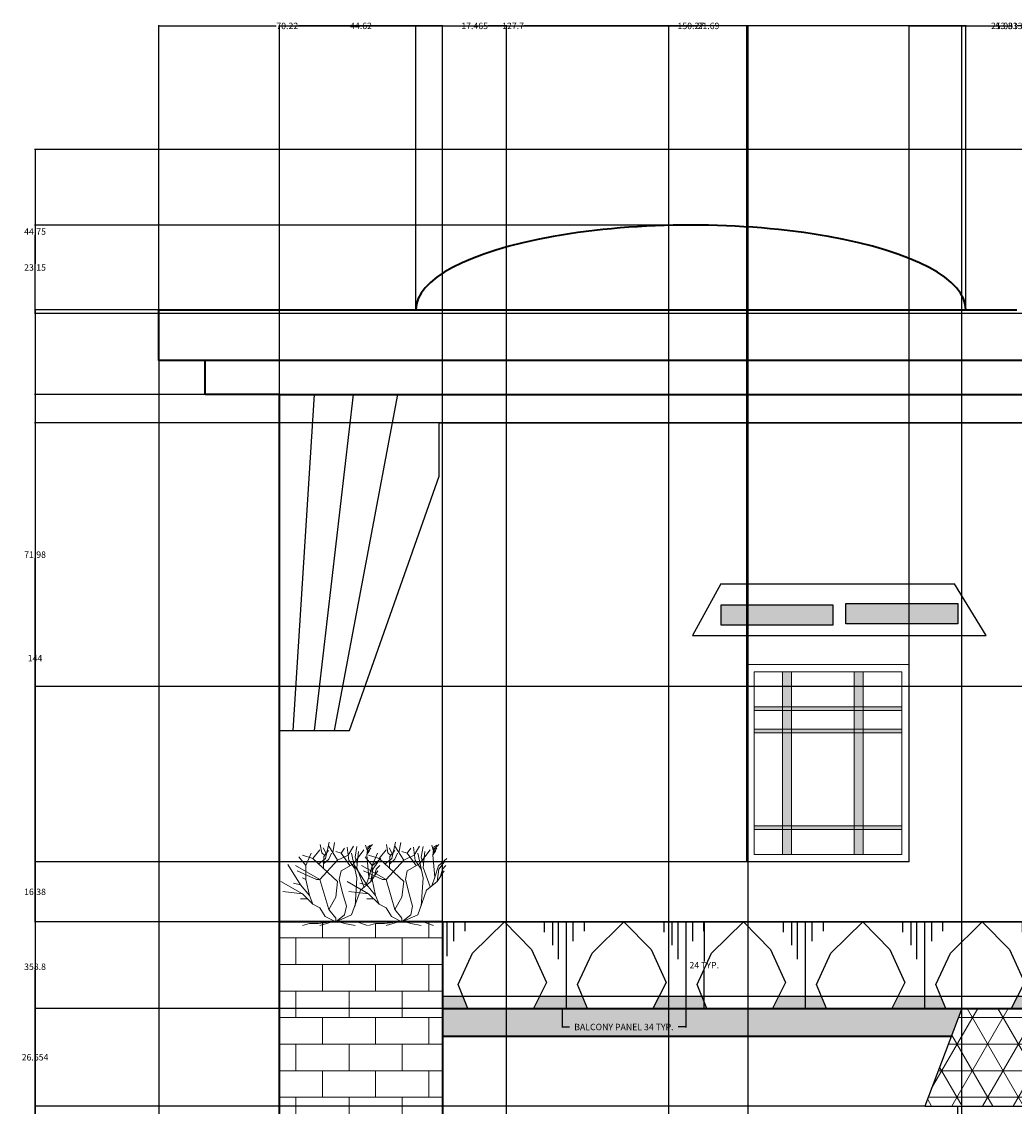
# Model space of a CAD drawing. Units: inches. Extents: x -17 to 741, y 7 to 490.
# Tile 2 of 8: x -17 to 254, y 193 to 490. Entities that reach past the tile are written whole.
import ezdxf

# ---------------------------------------------------------------- set-up
doc = ezdxf.new("R2010")
doc.units = ezdxf.units.IN
doc.header["$MEASUREMENT"] = 0
for name, color, linetype, lineweight in [('A-ANNO-DIMS', 2, 'Continuous', 18), ('A-ELEV-PATT', 252, 'Continuous', 13), ('A-FLOR-RAIL', 7, 'Continuous', 25), ('A-GLAZ', 4, 'Continuous', 18), ('A-ROOF', 7, 'Continuous', 35), ('A-ROOF-CNPE', 7, 'Continuous', 25), ('A-ROOF-PATT', 8, 'Continuous', 13), ('A-WALL', 7, 'Continuous', 35), ('A-WALL-PATT', 8, 'Continuous', 13), ('A-WALL-TRIM', 7, 'Continuous', 25), ('L-PLNT', 3, 'Continuous', 18)]:
    doc.layers.add(name, color=color, linetype=linetype, lineweight=lineweight)
doc.styles.get("Standard").update_dxf_attribs({"font": 'arial.ttf'})
doc.dimstyles.get("Standard").update_dxf_attribs({"dimtxt": 1.75, "dimasz": 0.18, "dimexe": 0.18, "dimexo": 0.0625, "dimgap": 0.09, "dimtad": 0, "dimtih": 1, "dimtoh": 1, "dimdec": 4, "dimzin": 0, "dimdsep": 46, "dimlunit": 4, "dimtxsty": 'Standard', "dimcen": 0.09, "dimadec": 0, "dimazin": 0, "dimtfac": 1, "dimtdec": 4, "dimtofl": 0, "dimtmove": 0, "dimatfit": 3, "dimfxl": 1, "dimtolj": 1, "dimtzin": 0, "dimarcsym": 0})

# ---------------------------------------------------------------- blocks, each defined once
blk = doc.blocks.new('Shrub - elevation')
for p, q in [((-12.471, 19.775), (-12.898, 22.044)), ((-11.28, 19.619), (-12.104, 21.184)), ((-11.433, 18.289), (-10.457, 22.749)), ((-8.16, 17.76), (-10.56, 21.6)), ((-9.48, 19.775), (-8.992, 22.592)), ((-7.2, 19.68), (-6.24, 21.12)), ((-5.086, 17.741), (-5.513, 21.34)), ((-5.28, 19.2), (-3.84, 21.6)), ((-3.377, 18.602), (-2.888, 21.575)), ((-0.508, 21.888), (-0.081, 20.558)), ((-0.203, 19.149), (0.102, 21.34)), ((-0.02, 20.01), (0.896, 21.105)), ((0.041, 20.714), (1.384, 22.044)), ((0.102, 21.34), (0.835, 21.888)), ((-16.8, 16.32), (-18.72, 18.72)), ((-14.88, 18.24), (-17.76, 19.2)), ((-16.8, 16.32), (-15.36, 19.68)), ((-14.88, 18.24), (-12.96, 20.64)), ((-8.16, 12), (-14.88, 18.24)), ((-13.325, 16.724), (-11.433, 18.289)), ((-11.677, 19.071), (-12.471, 19.775)), ((-12.043, 15.628), (-11.921, 18.836)), ((-11.982, 16.802), (-10.579, 18.054)), ((-11.921, 18.836), (-10.64, 20.401)), ((-10.579, 18.054), (-9.846, 19.697)), ((-7.2, 19.68), (-8.64, 20.16)), ((-8.16, 17.76), (-5.28, 19.2)), ((-4.8, 16.32), (-7.2, 19.68)), ((-3.377, 15.315), (-5.086, 17.819)), ((-2.88, 12.96), (-4.32, 19.68)), ((-3.84, 16.8), (-0.96, 20.64)), ((-2.766, 16.802), (-3.377, 18.602)), ((-2.88, 15.84), (-2.4, 20.16)), ((0.346, 13.203), (-0.203, 19.149)), ((-0.142, 19.384), (0.59, 20.401)), ((1.323, 16.254), (3.642, 18.289)), ((-18.24, 11.04), (-21.755, 16.655)), ((-12.96, 12.48), (-19.68, 16.32)), ((-13.92, 12.48), (-19.2, 14.88)), ((-16.8, 12.48), (-16.8, 16.32)), ((-12.96, 12.48), (-8.16, 17.76)), ((-7.68, 12.48), (-7.2, 14.88)), ((-7.2, 14.88), (-3.84, 16.8)), ((-0.96, 10.56), (-2.88, 15.84)), ((0.346, 13.203), (1.323, 16.254)), ((0.96, 12), (1.44, 15.36)), ((0.96, 12), (2.88, 14.88)), ((1.44, 15.36), (2.88, 17.28)), ((1.92, 13.44), (2.4, 15.36)), ((2.4, 15.36), (3.36, 16.32)), ((-17.76, 8.64), (-23.663, 11.961)), ((-16.8, 12.48), (-17.76, 12.96)), ((-15.84, 8.16), (-16.8, 12.48)), ((-12.96, 12.48), (-13.92, 12.48)), ((-10.56, 4.32), (-12.96, 12.48)), ((-8.64, 7.68), (-8.16, 12)), ((-6.72, 8.64), (-7.68, 12.48)), ((-3.36, 5.28), (-2.88, 12.96)), ((-1.92, 9.6), (0.96, 12)), ((-0.48, 10.8), (0.346, 13.203)), ((-17.76, 8.64), (-23.128, 9.222)), ((-18.24, 11.04), (-20.16, 11.52)), ((-15.84, 8.16), (-18.24, 11.04)), ((-4.32, 2.88), (-1.92, 9.6)), ((-16.32, 7.2), (-18.24, 7.2)), ((-14.88, 5.76), (-17.76, 8.64)), ((-14.88, 5.76), (-15.84, 8.16)), ((-10.56, 4.32), (-8.64, 7.68)), ((-5.76, 5.28), (-6.72, 8.64)), ((-12.96, 4.8), (-14.88, 5.76)), ((-11.52, 2.4), (-12.96, 4.8)), ((-8.64, 1.92), (-10.56, 4.32)), ((-6.24, 2.88), (-5.76, 5.28)), ((-15.84, 0.48), (-17.76, 0)), ((-13.44, 0.48), (-15.84, 0.48)), ((-9.6, 0.96), (-13.44, 0.48)), ((-9.6, 0.96), (-12.96, 0)), ((-8.64, 0.96), (-11.52, 2.4)), ((-9.6, 0.96), (-7.68, 0.96)), ((-8.64, 0.96), (-4.32, 2.88)), ((-8.64, 0.96), (-6.24, 2.88)), ((-8.64, 0.96), (-8.64, 1.92)), ((-8.64, 0.96), (-2.88, 0.96)), ((-7.68, 0.96), (-6.24, 0.48)), ((-6.24, 0.48), (-3.36, 0)), ((-2.88, 0.96), (0, 0))]:
    blk.add_line(p, q)
blk = doc.blocks.new('BALCONY-POINTED-PANEL')
for p, q in [((0, 23.66), (33.75, 23.66)), ((1.12, 23.66), (1.12, 14.33)), ((2.97, 23.66), (2.97, 18.36)), ((6.01, 23.66), (6.01, 21.09)), ((27.76, 23.66), (27.76, 20.83)), ((29.99, 23.66), (29.99, 17.32)), ((31.57, 23.66), (31.57, 13.51)), ((33.75, 23.66), (33.75, 0))]:
    blk.add_line(p, q)
blk.add_lwpolyline([(6.92, 0), (4.23, 6.57), (8.17, 15.14), (16.88, 23.66), (24.3, 16.07), (28.38, 7.1), (24.8, 0)])
blk = doc.blocks.new('WIN-ELEV-DIVIDED')
for p, q in [((9.78, 51.92), (9.78, 2)), ((12.23, 51.92), (12.23, 2)), ((29.29, 51.92), (29.29, 2)), ((31.75, 51.92), (31.75, 2)), ((2, 42.35), (42.31, 42.35)), ((2, 41.35), (42.31, 41.35)), ((2, 36.22), (42.31, 36.22)), ((2, 35.22), (42.31, 35.22)), ((2, 9.85), (42.31, 9.85)), ((2, 8.85), (42.31, 8.85))]:
    blk.add_line(p, q)
for points in [[(0, 0), (44.31, 0), (44.31, 53.92), (0, 53.92)], [(2, 2), (42.31, 2), (42.31, 51.92), (2, 51.92)]]:
    blk.add_lwpolyline(points, close=True)
blk = doc.blocks.new('*D15')
at = {"layer": 'A-ANNO-DIMS', "color": 0, "lineweight": -2, "transparency": 16777216}
for p, q in [((130.71, 219.95), (130.71, 214.77)), ((164.46, 219.95), (164.46, 214.77)), ((130.89, 214.95), (132.74, 214.95)), ((164.28, 214.95), (162.42, 214.95))]:
    blk.add_line(p, q, dxfattribs=at)
at = {"layer": 'A-ANNO-DIMS', "color": 0, "transparency": 16777216}
for points in [[(130.89, 214.98), (130.89, 214.92), (130.71, 214.95)], [(164.28, 214.98), (164.28, 214.92), (164.46, 214.95)]]:
    blk.add_solid(points, dxfattribs=at)
at = {"layer": 'Defpoints', "color": 0, "transparency": 16777216}
for p in [(130.71, 220.01), (164.46, 220.01), (164.46, 214.95)]:
    blk.add_point(p, dxfattribs=at)
at = {"layer": 'A-ANNO-DIMS', "color": 0, "transparency": 16777216, "insert": (147.58, 214.95), "char_height": 1.75, "attachment_point": 5}
blk.add_mtext('\\A1;BALCONY PANEL 34 TYP.', dxfattribs=at)
blk = doc.blocks.new('*D16')
at = {"layer": 'A-ANNO-DIMS', "color": 0, "lineweight": -2, "transparency": 16777216}
for p, q in [((164.52, 243.67), (169.7, 243.67)), ((169.52, 243.49), (169.52, 232.81)), ((169.52, 220.19), (169.52, 230.87)), ((164.52, 220.01), (169.7, 220.01))]:
    blk.add_line(p, q, dxfattribs=at)
at = {"layer": 'A-ANNO-DIMS', "color": 0, "transparency": 16777216}
for points in [[(169.49, 243.49), (169.55, 243.49), (169.52, 243.67)], [(169.49, 220.19), (169.55, 220.19), (169.52, 220.01)]]:
    blk.add_solid(points, dxfattribs=at)
at = {"layer": 'Defpoints', "color": 0, "transparency": 16777216}
for p in [(164.46, 243.67), (169.52, 243.67), (164.46, 220.01)]:
    blk.add_point(p, dxfattribs=at)
at = {"layer": 'A-ANNO-DIMS', "color": 0, "transparency": 16777216, "insert": (169.52, 231.84), "char_height": 1.75, "attachment_point": 5}
blk.add_mtext('\\A1;24 TYP.', dxfattribs=at)
blk = doc.blocks.new('*D37')
at = {"layer": 'A-ANNO-DIMS', "color": 0, "lineweight": -2, "transparency": 16777216}
for p, q in [((20.52, 396.95), (20.52, 14.58)), ((553.43, 51.95), (553.43, 14.58)), ((20.7, 14.76), (283.93, 14.76)), ((553.25, 14.76), (290.02, 14.76))]:
    blk.add_line(p, q, dxfattribs=at)
at = {"layer": 'A-ANNO-DIMS', "color": 0, "transparency": 16777216}
for points in [[(20.7, 14.79), (20.7, 14.73), (20.52, 14.76)], [(553.25, 14.79), (553.25, 14.73), (553.43, 14.76)]]:
    blk.add_solid(points, dxfattribs=at)
at = {"layer": 'Defpoints', "color": 0, "transparency": 16777216}
for p in [(20.52, 397.01), (553.43, 52.01), (553.43, 14.76)]:
    blk.add_point(p, dxfattribs=at)
at = {"layer": 'A-ANNO-DIMS', "color": 0, "transparency": 16777216, "insert": (286.97, 14.76), "char_height": 1.75, "attachment_point": 5}
blk.add_mtext('\\A1;532.9', dxfattribs=at)
blk = doc.blocks.new('*D39')
at = {"layer": 'A-ANNO-DIMS', "color": 0, "lineweight": -2, "transparency": 16777216}
for p, q in [((20.45, 410.82), (-13.46, 410.82)), ((-13.28, 410.64), (-13.28, 232.4)), ((-13.28, 52.19), (-13.28, 230.43)), ((53.4, 52.01), (-13.46, 52.01))]:
    blk.add_line(p, q, dxfattribs=at)
at = {"layer": 'A-ANNO-DIMS', "color": 0, "transparency": 16777216}
for points in [[(-13.31, 410.64), (-13.25, 410.64), (-13.28, 410.82)], [(-13.31, 52.19), (-13.25, 52.19), (-13.28, 52.01)]]:
    blk.add_solid(points, dxfattribs=at)
at = {"layer": 'Defpoints', "color": 0, "transparency": 16777216}
for p in [(-13.28, 410.82), (20.52, 410.82), (53.46, 52.01)]:
    blk.add_point(p, dxfattribs=at)
at = {"layer": 'A-ANNO-DIMS', "color": 0, "transparency": 16777216, "insert": (-13.28, 231.41), "char_height": 1.75, "attachment_point": 5}
blk.add_mtext('\\A1;358.8', dxfattribs=at)
blk = doc.blocks.new('*D40')
at = {"layer": 'A-ANNO-DIMS', "color": 0, "lineweight": -2, "transparency": 16777216}
for p, q in [((165.8, 433.97), (-13.46, 433.97)), ((-13.28, 433.79), (-13.28, 423.38)), ((-13.28, 411), (-13.28, 421.41)), ((90.67, 410.82), (-13.46, 410.82))]:
    blk.add_line(p, q, dxfattribs=at)
at = {"layer": 'A-ANNO-DIMS', "color": 0, "transparency": 16777216}
for points in [[(-13.31, 433.79), (-13.25, 433.79), (-13.28, 433.97)], [(-13.31, 411), (-13.25, 411), (-13.28, 410.82)]]:
    blk.add_solid(points, dxfattribs=at)
at = {"layer": 'Defpoints', "color": 0, "transparency": 16777216}
for p in [(-13.28, 433.97), (165.87, 433.97), (90.73, 410.82)]:
    blk.add_point(p, dxfattribs=at)
at = {"layer": 'A-ANNO-DIMS', "color": 0, "transparency": 16777216, "insert": (-13.28, 422.39), "char_height": 1.75, "attachment_point": 5}
blk.add_mtext('\\A1;23.15', dxfattribs=at)
blk = doc.blocks.new('*D41')
at = {"layer": 'A-ANNO-DIMS', "color": 0, "lineweight": -2, "transparency": 16777216}
for p, q in [((20.52, 410.88), (20.52, 488.55)), ((20.7, 488.37), (52.6, 488.37)), ((90.55, 488.37), (58.65, 488.37)), ((90.73, 410.88), (90.73, 488.55))]:
    blk.add_line(p, q, dxfattribs=at)
at = {"layer": 'A-ANNO-DIMS', "color": 0, "transparency": 16777216}
for points in [[(20.7, 488.4), (20.7, 488.34), (20.52, 488.37)], [(90.55, 488.4), (90.55, 488.34), (90.73, 488.37)]]:
    blk.add_solid(points, dxfattribs=at)
at = {"layer": 'Defpoints', "color": 0, "transparency": 16777216}
for p in [(90.73, 488.37), (20.52, 410.82), (90.73, 410.82)]:
    blk.add_point(p, dxfattribs=at)
at = {"layer": 'A-ANNO-DIMS', "color": 0, "transparency": 16777216, "insert": (55.62, 488.37), "char_height": 1.75, "attachment_point": 5}
blk.add_mtext('\\A1;70.22', dxfattribs=at)
blk = doc.blocks.new('*D42')
at = {"layer": 'A-ANNO-DIMS', "color": 0, "lineweight": -2, "transparency": 16777216}
for p, q in [((90.73, 410.88), (90.73, 488.55)), ((90.91, 488.37), (162.23, 488.37)), ((240.82, 488.37), (169.51, 488.37)), ((241, 410.88), (241, 488.55))]:
    blk.add_line(p, q, dxfattribs=at)
at = {"layer": 'A-ANNO-DIMS', "color": 0, "transparency": 16777216}
for points in [[(90.91, 488.4), (90.91, 488.34), (90.73, 488.37)], [(240.82, 488.4), (240.82, 488.34), (241, 488.37)]]:
    blk.add_solid(points, dxfattribs=at)
at = {"layer": 'Defpoints', "color": 0, "transparency": 16777216}
for p in [(241, 488.37), (90.73, 410.82), (241, 410.82)]:
    blk.add_point(p, dxfattribs=at)
at = {"layer": 'A-ANNO-DIMS', "color": 0, "transparency": 16777216, "insert": (165.87, 488.37), "char_height": 1.75, "attachment_point": 5}
blk.add_mtext('\\A1;150.27', dxfattribs=at)
blk = doc.blocks.new('*D43')
at = {"layer": 'A-ANNO-DIMS', "color": 0, "lineweight": -2, "transparency": 16777216}
for p, q in [((241, 410.88), (241, 488.55)), ((241.18, 488.37), (247.8, 488.37)), ((261.9, 488.37), (255.28, 488.37)), ((262.08, 409.88), (262.08, 488.55))]:
    blk.add_line(p, q, dxfattribs=at)
at = {"layer": 'A-ANNO-DIMS', "color": 0, "transparency": 16777216}
for points in [[(241.18, 488.4), (241.18, 488.34), (241, 488.37)], [(261.9, 488.4), (261.9, 488.34), (262.08, 488.37)]]:
    blk.add_solid(points, dxfattribs=at)
at = {"layer": 'Defpoints', "color": 0, "transparency": 16777216}
for p in [(262.08, 488.37), (241, 410.82), (262.08, 409.82)]:
    blk.add_point(p, dxfattribs=at)
at = {"layer": 'A-ANNO-DIMS', "color": 0, "transparency": 16777216, "insert": (251.54, 488.37), "char_height": 1.75, "attachment_point": 5}
blk.add_mtext('\\A1;21.083', dxfattribs=at)
blk = doc.blocks.new('*D45')
at = {"layer": 'A-ANNO-DIMS', "color": 0, "lineweight": -2, "transparency": 16777216}
for p, q in [((341.71, 454.57), (-13.46, 454.57)), ((-13.28, 454.39), (-13.28, 433.18)), ((-13.28, 410), (-13.28, 431.22)), ((262.02, 409.82), (-13.46, 409.82))]:
    blk.add_line(p, q, dxfattribs=at)
at = {"layer": 'A-ANNO-DIMS', "color": 0, "transparency": 16777216}
for points in [[(-13.31, 454.39), (-13.25, 454.39), (-13.28, 454.57)], [(-13.31, 410), (-13.25, 410), (-13.28, 409.82)]]:
    blk.add_solid(points, dxfattribs=at)
at = {"layer": 'Defpoints', "color": 0, "transparency": 16777216}
for p in [(-13.28, 454.57), (341.77, 454.57), (262.08, 409.82)]:
    blk.add_point(p, dxfattribs=at)
at = {"layer": 'A-ANNO-DIMS', "color": 0, "transparency": 16777216, "insert": (-13.28, 432.2), "char_height": 1.75, "attachment_point": 5}
blk.add_mtext('\\A1;44.75', dxfattribs=at)
blk = doc.blocks.new('*D47')
at = {"layer": 'A-ANNO-DIMS', "color": 0, "lineweight": -2, "transparency": 16777216}
for p, q in [((493.03, 379.95), (-13.46, 379.95)), ((-13.28, 379.77), (-13.28, 344.94)), ((-13.28, 308.15), (-13.28, 342.97)), ((553.37, 307.97), (-13.46, 307.97))]:
    blk.add_line(p, q, dxfattribs=at)
at = {"layer": 'A-ANNO-DIMS', "color": 0, "transparency": 16777216}
for points in [[(-13.31, 379.77), (-13.25, 379.77), (-13.28, 379.95)], [(-13.31, 308.15), (-13.25, 308.15), (-13.28, 307.97)]]:
    blk.add_solid(points, dxfattribs=at)
at = {"layer": 'Defpoints', "color": 0, "transparency": 16777216}
for p in [(493.1, 379.95), (-13.28, 307.97), (553.43, 307.97)]:
    blk.add_point(p, dxfattribs=at)
at = {"layer": 'A-ANNO-DIMS', "color": 0, "transparency": 16777216, "insert": (-13.28, 343.96), "char_height": 1.75, "attachment_point": 5}
blk.add_mtext('\\A1;71.98', dxfattribs=at)
blk = doc.blocks.new('*D49')
at = {"layer": 'A-ANNO-DIMS', "color": 0, "lineweight": -2, "transparency": 16777216}
for p, q in [((53.4, 243.67), (-13.46, 243.67)), ((-13.28, 243.49), (-13.28, 160.82)), ((-13.28, 76.19), (-13.28, 158.86)), ((53.4, 76.01), (-13.46, 76.01))]:
    blk.add_line(p, q, dxfattribs=at)
at = {"layer": 'A-ANNO-DIMS', "color": 0, "transparency": 16777216}
for points in [[(-13.31, 243.49), (-13.25, 243.49), (-13.28, 243.67)], [(-13.31, 76.19), (-13.25, 76.19), (-13.28, 76.01)]]:
    blk.add_solid(points, dxfattribs=at)
at = {"layer": 'Defpoints', "color": 0, "transparency": 16777216}
for p in [(-13.28, 243.67), (53.46, 243.67), (53.46, 76.01)]:
    blk.add_point(p, dxfattribs=at)
at = {"layer": 'A-ANNO-DIMS', "color": 0, "transparency": 16777216, "insert": (-13.28, 159.84), "char_height": 1.75, "attachment_point": 5}
blk.add_mtext('\\A1;167.66', dxfattribs=at)
blk = doc.blocks.new('*D50')
at = {"layer": 'A-ANNO-DIMS', "color": 0, "lineweight": -2, "transparency": 16777216}
for p, q in [((53.4, 387.67), (-13.46, 387.67)), ((-13.28, 387.49), (-13.28, 316.64)), ((-13.28, 243.85), (-13.28, 314.7)), ((53.4, 243.67), (-13.46, 243.67))]:
    blk.add_line(p, q, dxfattribs=at)
at = {"layer": 'A-ANNO-DIMS', "color": 0, "transparency": 16777216}
for points in [[(-13.31, 387.49), (-13.25, 387.49), (-13.28, 387.67)], [(-13.31, 243.85), (-13.25, 243.85), (-13.28, 243.67)]]:
    blk.add_solid(points, dxfattribs=at)
at = {"layer": 'Defpoints', "color": 0, "transparency": 16777216}
for p in [(-13.28, 387.67), (53.46, 387.67), (53.46, 243.67)]:
    blk.add_point(p, dxfattribs=at)
at = {"layer": 'A-ANNO-DIMS', "color": 0, "transparency": 16777216, "insert": (-13.28, 315.67), "char_height": 1.75, "attachment_point": 5}
blk.add_mtext('\\A1;144', dxfattribs=at)
blk = doc.blocks.new('*D51')
at = {"layer": 'A-ANNO-DIMS', "color": 0, "lineweight": -2, "transparency": 16777216}
for p, q in [((53.46, 52.07), (53.46, 488.55)), ((53.64, 488.37), (72.7, 488.37)), ((97.89, 488.37), (78.84, 488.37)), ((98.07, 52.07), (98.07, 488.55))]:
    blk.add_line(p, q, dxfattribs=at)
at = {"layer": 'A-ANNO-DIMS', "color": 0, "transparency": 16777216}
for points in [[(53.64, 488.4), (53.64, 488.34), (53.46, 488.37)], [(97.89, 488.4), (97.89, 488.34), (98.07, 488.37)]]:
    blk.add_solid(points, dxfattribs=at)
at = {"layer": 'Defpoints', "color": 0, "transparency": 16777216}
for p in [(98.07, 488.37), (53.46, 52.01), (98.07, 52.01)]:
    blk.add_point(p, dxfattribs=at)
at = {"layer": 'A-ANNO-DIMS', "color": 0, "transparency": 16777216, "insert": (75.77, 488.37), "char_height": 1.75, "attachment_point": 5}
blk.add_mtext('\\A1;44.62', dxfattribs=at)
blk = doc.blocks.new('*D52')
at = {"layer": 'A-ANNO-DIMS', "color": 0, "lineweight": -2, "transparency": 16777216}
for p, q in [((239.94, 113.25), (239.94, 488.55)), ((240.12, 488.37), (253.76, 488.37)), ((273.51, 488.37), (259.86, 488.37)), ((273.69, 113.25), (273.69, 488.55))]:
    blk.add_line(p, q, dxfattribs=at)
at = {"layer": 'A-ANNO-DIMS', "color": 0, "transparency": 16777216}
for points in [[(240.12, 488.4), (240.12, 488.34), (239.94, 488.37)], [(273.51, 488.4), (273.51, 488.34), (273.69, 488.37)]]:
    blk.add_solid(points, dxfattribs=at)
at = {"layer": 'Defpoints', "color": 0, "transparency": 16777216}
for p in [(273.69, 488.37), (239.94, 113.19), (273.69, 113.19)]:
    blk.add_point(p, dxfattribs=at)
at = {"layer": 'A-ANNO-DIMS', "color": 0, "transparency": 16777216, "insert": (256.81, 488.37), "char_height": 1.75, "attachment_point": 5}
blk.add_mtext('\\A1;33.75', dxfattribs=at)
blk = doc.blocks.new('*D55')
at = {"layer": 'A-ANNO-DIMS', "color": 0, "lineweight": -2, "transparency": 16777216}
for p, q in [((53.46, 243.73), (53.46, 488.55)), ((53.64, 488.37), (114.35, 488.37)), ((180.98, 488.37), (120.27, 488.37)), ((181.16, 260.11), (181.16, 488.55))]:
    blk.add_line(p, q, dxfattribs=at)
at = {"layer": 'A-ANNO-DIMS', "color": 0, "transparency": 16777216}
for points in [[(53.64, 488.4), (53.64, 488.34), (53.46, 488.37)], [(180.98, 488.4), (180.98, 488.34), (181.16, 488.37)]]:
    blk.add_solid(points, dxfattribs=at)
at = {"layer": 'Defpoints', "color": 0, "transparency": 16777216}
for p in [(181.16, 488.37), (181.16, 260.05), (53.46, 243.67)]:
    blk.add_point(p, dxfattribs=at)
at = {"layer": 'A-ANNO-DIMS', "color": 0, "transparency": 16777216, "insert": (117.31, 488.37), "char_height": 1.75, "attachment_point": 5}
blk.add_mtext('\\A1;127.7', dxfattribs=at)
blk = doc.blocks.new('*D56')
at = {"layer": 'A-ANNO-DIMS', "color": 0, "lineweight": -2, "transparency": 16777216}
for p, q in [((225.47, 260.11), (225.47, 488.55)), ((225.65, 488.37), (249.25, 488.37)), ((278.6, 488.37), (255, 488.37)), ((278.78, 243.73), (278.78, 488.55))]:
    blk.add_line(p, q, dxfattribs=at)
at = {"layer": 'A-ANNO-DIMS', "color": 0, "transparency": 16777216}
for points in [[(225.65, 488.4), (225.65, 488.34), (225.47, 488.37)], [(278.6, 488.4), (278.6, 488.34), (278.78, 488.37)]]:
    blk.add_solid(points, dxfattribs=at)
at = {"layer": 'Defpoints', "color": 0, "transparency": 16777216}
for p in [(278.78, 488.37), (225.47, 260.05), (278.78, 243.67)]:
    blk.add_point(p, dxfattribs=at)
at = {"layer": 'A-ANNO-DIMS', "color": 0, "transparency": 16777216, "insert": (252.12, 488.37), "char_height": 1.75, "attachment_point": 5}
blk.add_mtext('\\A1;53.31', dxfattribs=at)
blk = doc.blocks.new('*D58')
at = {"layer": 'A-ANNO-DIMS', "color": 0, "lineweight": -2, "transparency": 16777216}
for p, q in [((98.07, 52.07), (98.07, 488.55)), ((98.25, 488.37), (103.16, 488.37)), ((115.36, 488.37), (110.45, 488.37)), ((115.54, 153.67), (115.54, 488.55))]:
    blk.add_line(p, q, dxfattribs=at)
at = {"layer": 'A-ANNO-DIMS', "color": 0, "transparency": 16777216}
for points in [[(98.25, 488.4), (98.25, 488.34), (98.07, 488.37)], [(115.36, 488.4), (115.36, 488.34), (115.54, 488.37)]]:
    blk.add_solid(points, dxfattribs=at)
at = {"layer": 'Defpoints', "color": 0, "transparency": 16777216}
for p in [(115.54, 488.37), (115.54, 153.6), (98.07, 52.01)]:
    blk.add_point(p, dxfattribs=at)
at = {"layer": 'A-ANNO-DIMS', "color": 0, "transparency": 16777216, "insert": (106.81, 488.37), "char_height": 1.75, "attachment_point": 5}
blk.add_mtext('\\A1;17.465', dxfattribs=at)
blk = doc.blocks.new('*D59')
at = {"layer": 'A-ANNO-DIMS', "color": 0, "lineweight": -2, "transparency": 16777216}
for p, q in [((159.85, 153.67), (159.85, 488.55)), ((160.03, 488.37), (167.63, 488.37)), ((181.36, 488.37), (173.75, 488.37)), ((181.54, 153.67), (181.54, 488.55))]:
    blk.add_line(p, q, dxfattribs=at)
at = {"layer": 'A-ANNO-DIMS', "color": 0, "transparency": 16777216}
for points in [[(160.03, 488.4), (160.03, 488.34), (159.85, 488.37)], [(181.36, 488.4), (181.36, 488.34), (181.54, 488.37)]]:
    blk.add_solid(points, dxfattribs=at)
at = {"layer": 'Defpoints', "color": 0, "transparency": 16777216}
for p in [(181.54, 488.37), (159.85, 153.6), (181.54, 153.6)]:
    blk.add_point(p, dxfattribs=at)
at = {"layer": 'A-ANNO-DIMS', "color": 0, "transparency": 16777216, "insert": (170.69, 488.37), "char_height": 1.75, "attachment_point": 5}
blk.add_mtext('\\A1;21.69', dxfattribs=at)
blk = doc.blocks.new('*D62')
at = {"layer": 'A-ANNO-DIMS', "color": 0, "lineweight": -2, "transparency": 16777216}
for p, q in [((225.41, 260.05), (-13.46, 260.05)), ((-13.28, 259.87), (-13.28, 252.84)), ((-13.28, 243.85), (-13.28, 250.87)), ((278.72, 243.67), (-13.46, 243.67))]:
    blk.add_line(p, q, dxfattribs=at)
at = {"layer": 'A-ANNO-DIMS', "color": 0, "transparency": 16777216}
for points in [[(-13.31, 259.87), (-13.25, 259.87), (-13.28, 260.05)], [(-13.31, 243.85), (-13.25, 243.85), (-13.28, 243.67)]]:
    blk.add_solid(points, dxfattribs=at)
at = {"layer": 'Defpoints', "color": 0, "transparency": 16777216}
for p in [(225.47, 260.05), (-13.28, 243.67), (278.78, 243.67)]:
    blk.add_point(p, dxfattribs=at)
at = {"layer": 'A-ANNO-DIMS', "color": 0, "transparency": 16777216, "insert": (-13.28, 251.86), "char_height": 1.75, "attachment_point": 5}
blk.add_mtext('\\A1;16.38', dxfattribs=at)
blk = doc.blocks.new('*D66')
at = {"layer": 'A-ANNO-DIMS', "color": 0, "lineweight": -2, "transparency": 16777216}
for p, q in [((239.87, 220.01), (-13.46, 220.01)), ((-13.28, 219.83), (-13.28, 207.66)), ((-13.28, 193.53), (-13.28, 205.7)), ((229.69, 193.35), (-13.46, 193.35))]:
    blk.add_line(p, q, dxfattribs=at)
at = {"layer": 'A-ANNO-DIMS', "color": 0, "transparency": 16777216}
for points in [[(-13.31, 219.83), (-13.25, 219.83), (-13.28, 220.01)], [(-13.31, 193.53), (-13.25, 193.53), (-13.28, 193.35)]]:
    blk.add_solid(points, dxfattribs=at)
at = {"layer": 'Defpoints', "color": 0, "transparency": 16777216}
for p in [(-13.28, 220.01), (239.94, 220.01), (229.75, 193.35)]:
    blk.add_point(p, dxfattribs=at)
at = {"layer": 'A-ANNO-DIMS', "color": 0, "transparency": 16777216, "insert": (-13.28, 206.68), "char_height": 1.75, "attachment_point": 5}
blk.add_mtext('\\A1;26.654', dxfattribs=at)

msp = doc.modelspace()

# ---------------------------------------------------------------- hatches: boundary and pattern name
at = {"layer": 'A-ELEV-PATT'}
h = msp.add_hatch(dxfattribs=at)
h.set_pattern_fill('STARS', color=256, scale=19)
h.paths.add_polyline_path([(204.6793, 330.2905), (174.1219, 330.2905), (174.1219, 324.7204), (204.6793, 324.7204)])
h.paths.add_polyline_path([(238.7618, 330.6251), (208.2044, 330.6251), (208.2044, 325.055), (238.7618, 325.055)])
h.paths.add_polyline_path([(316.4391, 354.2167), (282.5434, 354.2167), (282.5434, 345.7496), (316.4391, 345.7496)])
h.paths.add_polyline_path([(360.3395, 354.2167), (326.4438, 354.2167), (326.4438, 345.7496), (360.3395, 345.7496)])
h.paths.add_polyline_path([(407.6938, 354.2167), (373.7981, 354.2167), (373.7981, 345.7496), (407.6938, 345.7496)])
h.paths.add_polyline_path([(290.7055, 188.3373), (256.8098, 188.3373), (256.8098, 179.8702), (290.7055, 179.8702)])
h.paths.add_polyline_path([(332.372, 188.3373), (298.4763, 188.3373), (298.4763, 179.8702), (332.372, 179.8702)])
h.paths.add_polyline_path([(375.4339, 188.3373), (341.5382, 188.3373), (341.5382, 179.8702), (375.4339, 179.8702)])
h.paths.add_polyline_path([(419.3343, 188.3373), (385.4386, 188.3373), (385.4386, 179.8702), (419.3343, 179.8702)])
h.paths.add_polyline_path([(466.6886, 188.3373), (432.7929, 188.3373), (432.7929, 179.8702), (466.6886, 179.8702)])
h = msp.add_hatch(color=256, dxfattribs=at)
h.dxf.hatch_style = 1
h.paths.add_polyline_path([(193.394, 295.2639), (190.938, 295.2639), (190.938, 269.8939), (193.394, 269.8939)])
h.paths.add_polyline_path([(193.394, 296.2639), (190.938, 296.2639), (190.938, 295.2639), (193.394, 295.2639)])
h.paths.add_polyline_path([(193.394, 311.9659), (190.938, 311.9659), (190.938, 296.2639), (193.394, 296.2639)])
h.paths.add_polyline_path([(190.938, 296.2639), (183.16, 296.2639), (183.16, 295.2639), (190.938, 295.2639)])
h.paths.add_polyline_path([(210.4499, 296.2639), (193.394, 296.2639), (193.394, 295.2639), (210.4499, 295.2639)])
h.paths.add_polyline_path([(212.9059, 311.9659), (210.4499, 311.9659), (210.4499, 296.2639), (212.9059, 296.2639)])
h.paths.add_polyline_path([(212.9059, 296.2639), (210.4499, 296.2639), (210.4499, 295.2639), (212.9059, 295.2639)])
h.paths.add_polyline_path([(223.4694, 296.2639), (212.9059, 296.2639), (212.9059, 295.2639), (223.4694, 295.2639)])
h.paths.add_polyline_path([(212.9059, 295.2639), (210.4499, 295.2639), (210.4499, 269.8939), (212.9059, 269.8939)])
h.paths.add_polyline_path([(193.394, 269.8939), (190.938, 269.8939), (190.938, 268.8939), (193.394, 268.8939)])
h.paths.add_polyline_path([(190.938, 269.8939), (183.16, 269.8939), (183.16, 268.8939), (190.938, 268.8939)])
h.paths.add_polyline_path([(210.4499, 269.8939), (193.394, 269.8939), (193.394, 268.8939), (210.4499, 268.8939)])
h.paths.add_polyline_path([(193.394, 268.8939), (190.938, 268.8939), (190.938, 262.0479), (193.394, 262.0479)])
h.paths.add_polyline_path([(212.9059, 269.8939), (210.4499, 269.8939), (210.4499, 268.8939), (212.9059, 268.8939)])
h.paths.add_polyline_path([(223.4694, 269.8939), (212.9059, 269.8939), (212.9059, 268.8939), (223.4694, 268.8939)])
h.paths.add_polyline_path([(212.9059, 268.8939), (210.4499, 268.8939), (210.4499, 262.0479), (212.9059, 262.0479)])
h.paths.add_polyline_path([(210.4499, 302.3991), (193.394, 302.3991), (193.394, 301.3991), (210.4499, 301.3991)])
h.paths.add_polyline_path([(223.4694, 302.3991), (212.9059, 302.3991), (212.9059, 301.3991), (223.4694, 301.3991)])
h.paths.add_polyline_path([(190.938, 302.3991), (183.16, 302.3991), (183.16, 301.3991), (190.938, 301.3991)])
h = msp.add_hatch(color=256, dxfattribs=at)
h.dxf.hatch_style = 1
h.paths.add_polyline_path([(103.6141, 223.3801), (98.075, 223.3801), (98.075, 220.0082), (104.992, 220.0082)])
h.paths.add_polyline_path([(131.8275, 223.3801), (124.5765, 223.3801), (122.878, 220.0082), (131.8275, 220.0082)])
h.paths.add_polyline_path([(136.2468, 223.3801), (131.8275, 223.3801), (131.8275, 220.0082), (137.6247, 220.0082)])
h.paths.add_polyline_path([(164.4602, 223.3801), (157.2092, 223.3801), (155.5107, 220.0082), (164.4602, 220.0082)])
h.paths.add_polyline_path([(168.8795, 223.3801), (164.4602, 223.3801), (164.4602, 220.0082), (170.2574, 220.0082)])
h.paths.add_polyline_path([(197.0929, 223.3801), (189.8419, 223.3801), (188.1434, 220.0082), (197.0929, 220.0082)])
h.paths.add_polyline_path([(201.5121, 223.3801), (197.0929, 223.3801), (197.0929, 220.0082), (202.8901, 220.0082)])
h.paths.add_polyline_path([(229.7256, 223.3801), (222.4746, 223.3801), (220.776, 220.0082), (229.7256, 220.0082)])
h.paths.add_polyline_path([(234.1448, 223.3801), (229.7256, 223.3801), (229.7256, 220.0082), (235.5227, 220.0082)])
h.paths.add_polyline_path([(262.3583, 223.3801), (255.1072, 223.3801), (253.4087, 220.0082), (262.3583, 220.0082)])
h.paths.add_polyline_path([(266.7775, 223.3801), (262.3583, 223.3801), (262.3583, 220.0082), (268.1554, 220.0082)])
h.paths.add_polyline_path([(294.9909, 223.3801), (287.7399, 223.3801), (286.0414, 220.0082), (294.9909, 220.0082)])
h.paths.add_polyline_path([(299.4102, 223.3801), (294.9909, 223.3801), (294.9909, 220.0082), (300.7881, 220.0082)])
h.paths.add_polyline_path([(327.6236, 223.3801), (320.3726, 223.3801), (318.6741, 220.0082), (327.6236, 220.0082)])
h.paths.add_polyline_path([(332.0429, 223.3801), (327.6236, 223.3801), (327.6236, 220.0082), (333.4208, 220.0082)])
h.paths.add_polyline_path([(360.2563, 223.3801), (353.0053, 223.3801), (351.3068, 220.0082), (360.2563, 220.0082)])
h.paths.add_polyline_path([(364.6755, 223.3801), (360.2563, 223.3801), (360.2563, 220.0082), (361.2234, 220.0082), (366.0535, 220.0082)])
h.paths.add_polyline_path([(392.889, 223.3801), (385.638, 223.3801), (383.9394, 220.0082), (392.889, 220.0082)])
h.paths.add_polyline_path([(397.3082, 223.3801), (392.889, 223.3801), (392.889, 220.0082), (398.6861, 220.0082)])
h.paths.add_polyline_path([(425.5216, 223.3801), (418.2706, 223.3801), (416.5721, 220.0082), (425.5216, 220.0082)])
h.paths.add_polyline_path([(429.9409, 223.3801), (425.5216, 223.3801), (425.5216, 220.0082), (431.3188, 220.0082)])
h.paths.add_polyline_path([(458.1543, 223.3801), (450.9033, 223.3801), (449.2048, 220.0082), (458.1543, 220.0082)])
at = {"layer": 'A-ROOF-PATT'}
h = msp.add_hatch(dxfattribs=at)
h.set_pattern_fill('NET3', color=256, scale=58)
h.paths.add_polyline_path([(478.3168, 220.0082), (470.3932, 220.0082), (361.2234, 220.0082), (239.9367, 220.0082), (229.7523, 193.3539), (470.754, 193.3539), (488.0578, 193.3539)])
h.paths.add_polyline_path([(421.4932, 379.9466), (278.7803, 379.9466), (278.7803, 359.2334), (411.7592, 359.2334), (429.063, 359.2334)])
at = {"layer": 'A-WALL-PATT'}
h = msp.add_hatch(dxfattribs=at)
h.set_pattern_fill('BRICK', color=256, scale=29)
h.paths.add_polyline_path([(98.075, 232.0082), (98.075, 243.669), (86.0039, 243.669), (82.1639, 243.189), (79.7639, 243.189), (77.6592, 242.6628), (74.6406, 243.669), (68.8806, 243.669), (67.9206, 243.669), (53.4591, 243.669), (53.4591, 220.0082), (53.4591, 76.0082), (98.075, 76.0082)])
h = msp.add_hatch(dxfattribs=at)
h.set_pattern_fill('EARTH', color=256, scale=13, angle=16)
h.paths.add_polyline_path([(273.6893, 89.5255), (239.9367, 89.5255), (239.9367, 76.0082), (273.6893, 76.0082)])
h.paths.add_polyline_path([(394.976, 89.5255), (361.2234, 89.5255), (361.2234, 76.0082), (394.976, 76.0082)])
h.paths.add_polyline_path([(428.7285, 89.5255), (394.976, 89.5255), (394.976, 76.0082), (428.7285, 76.0082)])
h.paths.add_polyline_path([(460.302, 89.5255), (428.7285, 89.5255), (428.7285, 76.0082), (460.302, 76.0082)])
h.paths.add_polyline_path([(239.9367, 220.0082), (98.075, 220.0082), (98.075, 212.3604), (237.0146, 212.3604)])

# ---------------------------------------------------------------- linework, layer by layer
at = {"layer": 'A-FLOR-RAIL'}
for p, q in [((98.075, 223.3801), (478.3168, 223.3801)), ((98.075, 220.0082), (131.8275, 220.0082))]:
    msp.add_line(p, q, dxfattribs=at)
at = {"layer": 'A-ROOF'}
for p, q in [((20.5169, 397.0087), (20.5169, 410.8173)), ((20.5169, 410.8173), (254.8926, 410.8173)), ((258.4874, 397.0087), (20.5169, 397.0087)), ((33.1823, 395.4079), (33.1823, 397.0087)), ((33.1823, 387.669), (33.1823, 395.4079)), ((53.4591, 387.669), (33.1823, 387.669)), ((53.4591, 387.669), (421.4932, 387.669)), ((53.4591, 363.669), (53.4591, 387.669))]:
    msp.add_line(p, q, dxfattribs=at)
msp.add_ellipse((165.8655, 410.8173), major_axis=(-75.1331, 0), ratio=0.30809711, start_param=3.14159265, end_param=6.28318531, dxfattribs=at)
at = {"layer": 'A-ROOF-CNPE'}
for p, q in [((174.0468, 336.0024), (237.8913, 336.0024)), ((238.7685, 190.3139), (238.7685, 193.3539))]:
    msp.add_line(p, q, dxfattribs=at)
for points in [[(174.0468, 336.0024), (166.3147, 321.8751), (246.507, 321.8751), (237.8913, 336.0024)], [(239.9367, 220.0082), (229.7523, 193.3539), (470.754, 193.3539)]]:
    msp.add_lwpolyline(points, dxfattribs=at)
for points in [[(174.1219, 330.2905), (204.6793, 330.2905), (204.6793, 324.7204), (174.1219, 324.7204)], [(208.2044, 330.6251), (238.7618, 330.6251), (238.7618, 325.055), (208.2044, 325.055)]]:
    msp.add_lwpolyline(points, close=True, dxfattribs=at)
at = {"layer": 'A-WALL'}
for p, q in [((53.4591, 243.669), (53.4591, 363.669)), ((53.4591, 220.0082), (53.4591, 243.669)), ((98.075, 243.669), (53.4591, 243.669)), ((98.075, 232.0082), (98.075, 243.669)), ((98.075, 52.0082), (98.075, 232.0082)), ((53.4591, 76.0082), (53.4591, 220.0082)), ((98.075, 220.0082), (361.2234, 220.0082)), ((237.0146, 212.3604), (98.075, 212.3604))]:
    msp.add_line(p, q, dxfattribs=at)
at = {"layer": 'A-WALL-TRIM'}
for p, q in [((57.1971, 295.9), (63.1007, 387.669)), ((63.0342, 295.9), (73.7245, 387.669)), ((68.5662, 295.9), (85.8252, 387.669))]:
    msp.add_line(p, q, dxfattribs=at)
msp.add_lwpolyline([(53.4591, 295.9), (53.4591, 295.9), (72.6093, 295.9), (97.1425, 365.3552), (97.1425, 379.9466), (515.96, 379.9466)], dxfattribs=at)

# ---------------------------------------------------------------- block references
at = {"layer": 'A-FLOR-RAIL'}
for p in [(98.075, 220.008), (130.7077, 220.008), (163.3404, 220.008), (195.973, 220.008), (228.6057, 220.008)]:
    msp.add_blockref('BALCONY-POINTED-PANEL', p, dxfattribs=at)
at = {"layer": 'A-GLAZ'}
msp.add_blockref('WIN-ELEV-DIVIDED', (181.16, 260.048), dxfattribs=at)
at = {"layer": 'L-PLNT'}
for p in [(77.5206, 242.709), (95.6039, 242.709)]:
    msp.add_blockref('Shrub - elevation', p, dxfattribs=at)

# ---------------------------------------------------------------- dimensions: what is measured, and where the dimension line sits
at = {"layer": 'A-ANNO-DIMS'}
for base, p1, p2, override, picture, middle in [((90.7324, 488.3717), (20.5169, 410.8173), (90.7324, 410.8173), {"dimdec": 2, "dimlfac": 1, "dimrnd": 0, "dimzin": 0, "dimdsep": 46, "dimlunit": 2}, '*D41', (55.6246, 488.3717)), ((98.075, 488.3717), (53.4591, 52.0082), (98.075, 52.0082), {"dimdec": 2, "dimlfac": 1, "dimrnd": 0, "dimzin": 0, "dimdsep": 46, "dimlunit": 2}, '*D51', (75.7671, 488.3717)), ((181.16, 488.3717), (53.4591, 243.669), (181.16, 260.0479), {"dimdec": 1, "dimlfac": 1, "dimrnd": 0, "dimzin": 0, "dimdsep": 46, "dimlunit": 2}, '*D55', (117.3096, 488.3717)), ((240.9987, 488.3717), (90.7324, 410.8173), (240.9987, 410.8173), {"dimdec": 2, "dimlfac": 1, "dimrnd": 0, "dimzin": 0, "dimdsep": 46, "dimlunit": 2}, '*D42', (165.8655, 488.3717)), ((115.54046, 488.37169), (98.07499, 52.00816), (115.54046, 153.60279), {"dimdec": 3, "dimlfac": 1, "dimrnd": 0, "dimzin": 0, "dimdsep": 46, "dimlunit": 2}, '*D58', (106.80773, 488.37169)), ((181.5379, 488.3717), (159.8499, 153.6028), (181.5379, 153.6028), {"dimdec": 2, "dimlfac": 1, "dimrnd": 0, "dimzin": 0, "dimdsep": 46, "dimlunit": 2}, '*D59', (170.6939, 488.3717)), ((278.7803, 488.3717), (225.4694, 260.0479), (278.7803, 243.669), {"dimdec": 2, "dimlfac": 1, "dimrnd": 0, "dimzin": 0, "dimdsep": 46, "dimlunit": 2}, '*D56', (252.1249, 488.3717)), ((273.6893, 488.3717), (239.9367, 113.1863), (273.6893, 113.1863), {"dimdec": 2, "dimlfac": 1, "dimrnd": 0, "dimzin": 0, "dimdsep": 46, "dimlunit": 2}, '*D52', (256.813, 488.3717)), ((262.0821, 488.3717), (240.9987, 410.8173), (262.0821, 409.8217), {"dimdec": 3, "dimlfac": 1, "dimrnd": 0, "dimzin": 0, "dimdsep": 46, "dimlunit": 2}, '*D43', (251.5404, 488.3717)), ((553.4286, 14.7597), (20.5169, 397.0087), (553.4286, 52.0082), {"dimdec": 1, "dimlfac": 1, "dimrnd": 0, "dimzin": 0, "dimdsep": 46, "dimlunit": 2}, '*D37', (286.9727, 14.7597))]:
    dim = msp.add_linear_dim(base=base, p1=p1, p2=p2, dimstyle='Standard', override=override, dxfattribs=at)
    dim.commit()
    dim.dimension.update_dxf_attribs({"geometry": picture, "text_midpoint": middle})
for base, p1, p2, override, picture, middle in [((-13.2831, 454.5717), (262.0821, 409.8217), (341.7687, 454.5717), {"dimdec": 2, "dimlfac": 1, "dimrnd": 0, "dimzin": 0, "dimdsep": 46, "dimlunit": 2}, '*D45', (-13.2831, 432.1967)), ((-13.2831, 433.9656), (90.7324, 410.8173), (165.8655, 433.9656), {"dimdec": 2, "dimlfac": 1, "dimrnd": 0, "dimzin": 0, "dimdsep": 46, "dimlunit": 2}, '*D40', (-13.2831, 422.3914)), ((-13.2831, 410.8173), (53.4591, 52.0082), (20.5169, 410.8173), {"dimdec": 1, "dimlfac": 1, "dimrnd": 0, "dimzin": 0, "dimdsep": 46, "dimlunit": 2}, '*D39', (-13.2831, 231.4127)), ((-13.2831, 387.669), (53.4591, 243.669), (53.4591, 387.669), {"dimdec": 0, "dimlfac": 1, "dimrnd": 0, "dimzin": 0, "dimdsep": 46, "dimlunit": 2}, '*D50', (-13.2831, 315.669)), ((-13.2831, 307.9703), (493.0961, 379.9466), (553.4286, 307.9703), {"dimdec": 2, "dimlfac": 1, "dimrnd": 0, "dimzin": 0, "dimdsep": 46, "dimlunit": 2}, '*D47', (-13.2831, 343.9584)), ((-13.2831, 243.669), (225.4694, 260.0479), (278.7803, 243.669), {"dimdec": 2, "dimlfac": 1, "dimrnd": 0, "dimzin": 0, "dimdsep": 46, "dimlunit": 2}, '*D62', (-13.2831, 251.8584)), ((-13.2831, 243.669), (53.4591, 76.0082), (53.4591, 243.669), {"dimdec": 2, "dimlfac": 1, "dimrnd": 0, "dimzin": 0, "dimdsep": 46, "dimlunit": 2}, '*D49', (-13.2831, 159.8386)), ((-13.2831, 220.0082), (229.7523, 193.3539), (239.9367, 220.0082), {"dimdec": 3, "dimlfac": 1, "dimrnd": 0, "dimzin": 0, "dimdsep": 46, "dimlunit": 2}, '*D66', (-13.2831, 206.681))]:
    dim = msp.add_linear_dim(base=base, p1=p1, p2=p2, angle=90, dimstyle='Standard', override=override, dxfattribs=at)
    dim.commit()
    dim.dimension.update_dxf_attribs({"geometry": picture, "text_midpoint": middle})
dim = msp.add_linear_dim(base=(169.5231, 243.669), p1=(164.4602, 220.0082), p2=(164.4602, 243.669), angle=90, text='<> TYP.', dimstyle='Standard', override={"dimdec": 0, "dimlfac": 1, "dimrnd": 0, "dimzin": 0, "dimdsep": 46, "dimlunit": 2}, dxfattribs=at)
dim.commit()
dim.dimension.update_dxf_attribs({"geometry": '*D16', "text_midpoint": (169.5231, 231.8386)})
dim = msp.add_linear_dim(base=(164.4602, 214.9453), p1=(130.7077, 220.0082), p2=(164.4602, 220.0082), text='BALCONY PANEL <> TYP.', dimstyle='Standard', override={"dimdec": 0, "dimlfac": 1, "dimrnd": 0, "dimzin": 0, "dimdsep": 46, "dimlunit": 2}, dxfattribs=at)
dim.commit()
dim.dimension.update_dxf_attribs({"geometry": '*D15', "text_midpoint": (147.5839, 214.9453)})

doc.saveas('drawing.dxf')
